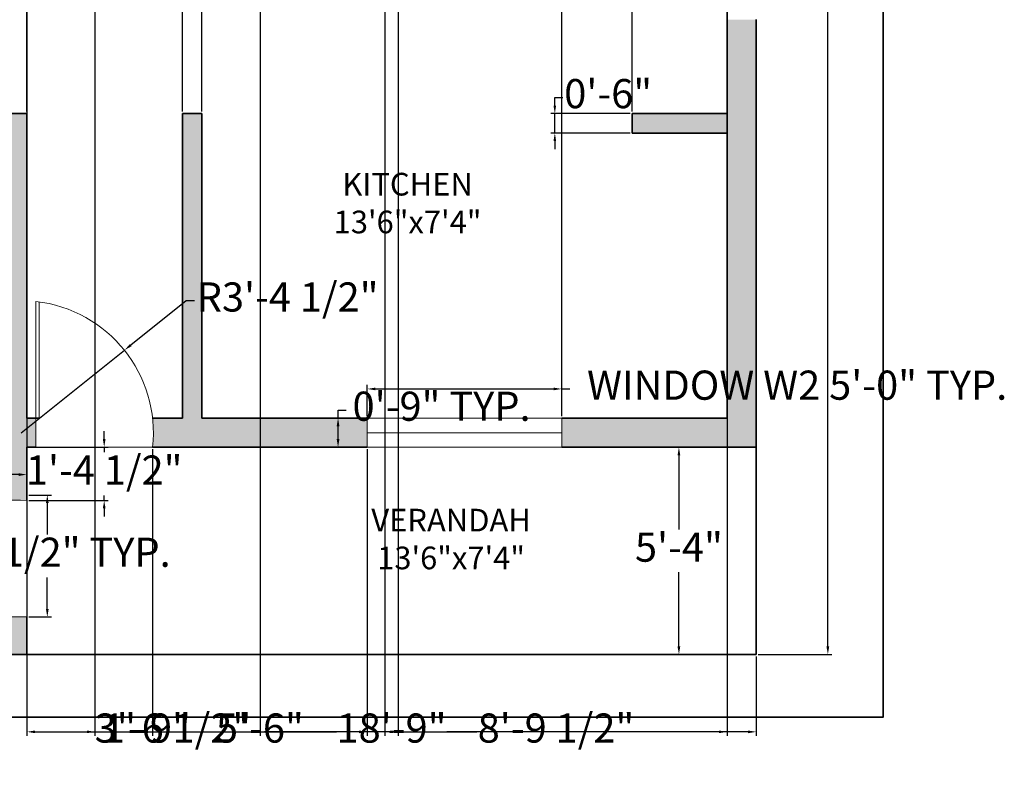
# Model space of a CAD drawing. Units: inches. Extents: x 2151 to 2709, y 3533 to 4046.
# Tile 3 of 4: x 2406 to 2709, y 3533 to 3766. Entities that reach past the tile are written whole.
import ezdxf

# ---------------------------------------------------------------- set-up
doc = ezdxf.new("R2010")
doc.units = ezdxf.units.IN
for name, color, linetype, lineweight in [('A-ANNO-DIMS', 2, 'Continuous', 18), ('A-ANNO-TTLB', 7, 'Continuous', 35), ('A-AREA-IDEN', 7, 'Continuous', 25), ('A-DOOR', 3, 'Continuous', 18), ('A-GLAZ', 4, 'Continuous', 18), ('A-WALL', 7, 'Continuous', 35)]:
    doc.layers.add(name, color=color, linetype=linetype, lineweight=lineweight)
doc.layers.add('A-WALL-PATT', color=18, linetype='Continuous', lineweight=13, true_color=0x000000)
doc.styles.get("Standard").update_dxf_attribs({"font": 'arial.ttf'})
doc.dimstyles.new('ISO-25', dxfattribs={"dimtxt": 9, "dimasz": 2.5, "dimexe": 1.25, "dimexo": 0.625, "dimgap": 2, "dimtad": 0, "dimtih": 1, "dimtoh": 1, "dimdec": 1, "dimlunit": 4, "dimtxsty": 'Standard', "dimcen": 2.5, "dimadec": 0, "dimazin": 0, "dimtfac": 0.5, "dimtdec": 1, "dimtmove": 0, "dimatfit": 3, "dimfxl": 1, "dimarcsym": 0})

# ---------------------------------------------------------------- blocks, each defined once
blk = doc.blocks.new('*D7')
at = {"layer": 'A-ANNO-DIMS', "color": 0, "lineweight": -2, "transparency": 16777216}
for p, q in [((2633.46, 4002.17), (2656.18, 4002.17)), ((2654.93, 3999.67), (2654.93, 3792.76)), ((2654.93, 3572.67), (2654.93, 3779.57)), ((2633.46, 3570.17), (2656.18, 3570.17))]:
    blk.add_line(p, q, dxfattribs=at)
at = {"layer": 'A-ANNO-DIMS', "color": 0, "transparency": 16777216}
for points in [[(2654.51, 3999.67), (2655.35, 3999.67), (2654.93, 4002.17)], [(2654.51, 3572.67), (2655.35, 3572.67), (2654.93, 3570.17)]]:
    blk.add_solid(points, dxfattribs=at)
at = {"layer": 'Defpoints', "color": 0, "transparency": 16777216}
for p in [(2632.83, 4002.17), (2632.83, 3570.17), (2654.93, 3570.17)]:
    blk.add_point(p, dxfattribs=at)
at = {"layer": 'A-ANNO-DIMS', "color": 0, "transparency": 16777216, "insert": (2654.93, 3786.17), "char_height": 9, "attachment_point": 5}
blk.add_mtext("36'", dxfattribs=at)
blk = doc.blocks.new('WIN-60IN')
for p, q in [((0, 9), (0, 0)), ((0, 9), (60, 9)), ((60, 9), (60, 0)), ((0, 4.5), (60, 4.5)), ((0, 0), (60, 0))]:
    blk.add_line(p, q)
blk = doc.blocks.new('DOOR-SWING-36IN')
for p, q in [((0, 6), (0, 42)), ((1, 6), (1, 41.91)), ((0, 6), (0, 0)), ((0, 0), (36, 0))]:
    blk.add_line(p, q)
blk.add_arc((-3, 3), 39.12, 355.6013, 85.6013)
blk = doc.blocks.new('*D15')
at = {"layer": 'A-ANNO-DIMS', "color": 0, "lineweight": -2, "transparency": 16777216}
for p, q in [((2512.83, 3643.79), (2512.83, 3653.42)), ((2515.33, 3652.17), (2570.33, 3652.17)), ((2572.83, 3643.79), (2572.83, 3653.42)), ((2572.83, 3652.17), (2575.33, 3652.17))]:
    blk.add_line(p, q, dxfattribs=at)
at = {"layer": 'A-ANNO-DIMS', "color": 0, "transparency": 16777216}
for points in [[(2515.33, 3652.58), (2515.33, 3651.75), (2512.83, 3652.17)], [(2570.33, 3652.58), (2570.33, 3651.75), (2572.83, 3652.17)]]:
    blk.add_solid(points, dxfattribs=at)
at = {"layer": 'Defpoints', "color": 0, "transparency": 16777216}
for p in [(2572.83, 3652.17), (2512.83, 3643.17), (2572.83, 3643.17)]:
    blk.add_point(p, dxfattribs=at)
at = {"layer": 'A-ANNO-DIMS', "color": 0, "transparency": 16777216, "insert": (2645.45, 3652.17), "char_height": 9, "attachment_point": 5}
blk.add_mtext('WINDOW W2 5\'-0" TYP.', dxfattribs=at)
blk = doc.blocks.new('*D16')
at = {"layer": 'A-ANNO-DIMS', "color": 0, "lineweight": -2, "transparency": 16777216}
for p, q in [((2503.83, 3643.17), (2503.83, 3645.67)), ((2503.83, 3645.67), (2506.33, 3645.67)), ((2512.21, 3643.17), (2502.58, 3643.17)), ((2503.83, 3636.67), (2503.83, 3640.67)), ((2512.21, 3634.17), (2502.58, 3634.17))]:
    blk.add_line(p, q, dxfattribs=at)
at = {"layer": 'A-ANNO-DIMS', "color": 0, "transparency": 16777216}
for points in [[(2503.41, 3640.67), (2504.25, 3640.67), (2503.83, 3643.17)], [(2503.41, 3636.67), (2504.25, 3636.67), (2503.83, 3634.17)]]:
    blk.add_solid(points, dxfattribs=at)
at = {"layer": 'Defpoints', "color": 0, "transparency": 16777216}
for p in [(2503.83, 3643.17), (2512.83, 3643.17), (2512.83, 3634.17)]:
    blk.add_point(p, dxfattribs=at)
at = {"layer": 'A-ANNO-DIMS', "color": 0, "transparency": 16777216, "insert": (2535.76, 3645.67), "char_height": 9, "attachment_point": 5}
blk.add_mtext('0\'-9" TYP.', dxfattribs=at)
blk = doc.blocks.new('*D17')
at = {"layer": 'A-ANNO-DIMS', "color": 0, "lineweight": -2, "transparency": 16777216}
for p, q in [((2365.83, 3620.05), (2365.83, 3626.98)), ((2407.83, 3620.05), (2407.83, 3626.98)), ((2365.83, 3625.73), (2363.33, 3625.73)), ((2405.33, 3625.73), (2368.33, 3625.73))]:
    blk.add_line(p, q, dxfattribs=at)
at = {"layer": 'A-ANNO-DIMS', "color": 0, "transparency": 16777216}
for points in [[(2368.33, 3626.14), (2368.33, 3625.31), (2365.83, 3625.73)], [(2405.33, 3626.14), (2405.33, 3625.31), (2407.83, 3625.73)]]:
    blk.add_solid(points, dxfattribs=at)
at = {"layer": 'Defpoints', "color": 0, "transparency": 16777216}
for p in [(2365.83, 3625.73), (2365.83, 3619.43), (2407.83, 3619.43)]:
    blk.add_point(p, dxfattribs=at)
at = {"layer": 'A-ANNO-DIMS', "color": 0, "transparency": 16777216, "insert": (2303.74, 3625.73), "char_height": 9, "attachment_point": 5}
blk.add_mtext('DOOR D1 3\'-6" TYP.', dxfattribs=at)
blk = doc.blocks.new('*D18')
at = {"layer": 'A-ANNO-DIMS', "color": 0, "lineweight": -2, "transparency": 16777216}
for p, q in [((2408.46, 3619.43), (2415.38, 3619.43)), ((2414.13, 3616.93), (2414.13, 3607.26)), ((2414.13, 3584.27), (2414.13, 3593.94)), ((2408.46, 3581.77), (2415.38, 3581.77))]:
    blk.add_line(p, q, dxfattribs=at)
at = {"layer": 'A-ANNO-DIMS', "color": 0, "transparency": 16777216}
for points in [[(2413.71, 3616.93), (2414.55, 3616.93), (2414.13, 3619.43)], [(2413.71, 3584.27), (2414.55, 3584.27), (2414.13, 3581.77)]]:
    blk.add_solid(points, dxfattribs=at)
at = {"layer": 'Defpoints', "color": 0, "transparency": 16777216}
for p in [(2407.83, 3619.43), (2414.13, 3619.43), (2407.83, 3581.77)]:
    blk.add_point(p, dxfattribs=at)
at = {"layer": 'A-ANNO-DIMS', "color": 0, "transparency": 16777216, "insert": (2414.13, 3600.6), "char_height": 9, "attachment_point": 5}
blk.add_mtext('3\'-1 1/2" TYP.', dxfattribs=at)
blk = doc.blocks.new('*D25')
at = {"layer": 'A-ANNO-DIMS', "color": 0, "lineweight": -2, "transparency": 16777216}
for p, q in [((2407.83, 3737.79), (2407.83, 4027.27)), ((2410.33, 4026.02), (2417.69, 4026.02)), ((2453.33, 4026.02), (2445.97, 4026.02)), ((2455.83, 3737.79), (2455.83, 4027.27))]:
    blk.add_line(p, q, dxfattribs=at)
at = {"layer": 'A-ANNO-DIMS', "color": 0, "transparency": 16777216}
for points in [[(2410.33, 4026.43), (2410.33, 4025.6), (2407.83, 4026.02)], [(2453.33, 4026.43), (2453.33, 4025.6), (2455.83, 4026.02)]]:
    blk.add_solid(points, dxfattribs=at)
at = {"layer": 'Defpoints', "color": 0, "transparency": 16777216}
for p in [(2455.83, 4026.02), (2407.83, 3737.17), (2455.83, 3737.17)]:
    blk.add_point(p, dxfattribs=at)
at = {"layer": 'A-ANNO-DIMS', "color": 0, "transparency": 16777216, "insert": (2431.83, 4026.02), "char_height": 9, "attachment_point": 5}
blk.add_mtext('4\'-0"', dxfattribs=at)
blk = doc.blocks.new('*D26')
at = {"layer": 'A-ANNO-DIMS', "color": 0, "lineweight": -2, "transparency": 16777216}
for p, q in [((2570.7, 3739.67), (2570.7, 3742.17)), ((2570.7, 3742.17), (2573.2, 3742.17)), ((2593.92, 3737.17), (2569.45, 3737.17)), ((2570.7, 3731.17), (2570.7, 3737.17)), ((2593.92, 3731.17), (2569.45, 3731.17)), ((2570.7, 3728.67), (2570.7, 3726.17))]:
    blk.add_line(p, q, dxfattribs=at)
at = {"layer": 'A-ANNO-DIMS', "color": 0, "transparency": 16777216}
for points in [[(2570.28, 3739.67), (2571.11, 3739.67), (2570.7, 3737.17)], [(2570.28, 3728.67), (2571.11, 3728.67), (2570.7, 3731.17)]]:
    blk.add_solid(points, dxfattribs=at)
at = {"layer": 'Defpoints', "color": 0, "transparency": 16777216}
for p in [(2570.7, 3737.17), (2594.55, 3737.17), (2594.55, 3731.17)]:
    blk.add_point(p, dxfattribs=at)
at = {"layer": 'A-ANNO-DIMS', "color": 0, "transparency": 16777216, "insert": (2587.16, 3742.17), "char_height": 9, "attachment_point": 5}
blk.add_mtext('0\'-6"', dxfattribs=at)
blk = doc.blocks.new('*D27')
at = {"layer": 'A-ANNO-DIMS', "color": 0, "lineweight": -2, "transparency": 16777216}
for p, q in [((2632.21, 3634.17), (2607.73, 3634.17)), ((2608.98, 3631.67), (2608.98, 3608.74)), ((2608.98, 3572.67), (2608.98, 3595.59)), ((2632.21, 3570.17), (2607.73, 3570.17))]:
    blk.add_line(p, q, dxfattribs=at)
at = {"layer": 'A-ANNO-DIMS', "color": 0, "transparency": 16777216}
for points in [[(2608.56, 3631.67), (2609.4, 3631.67), (2608.98, 3634.17)], [(2608.56, 3572.67), (2609.4, 3572.67), (2608.98, 3570.17)]]:
    blk.add_solid(points, dxfattribs=at)
at = {"layer": 'Defpoints', "color": 0, "transparency": 16777216}
for p in [(2608.98, 3634.17), (2632.83, 3634.17), (2632.83, 3570.17)]:
    blk.add_point(p, dxfattribs=at)
at = {"layer": 'A-ANNO-DIMS', "color": 0, "transparency": 16777216, "insert": (2608.98, 3602.17), "char_height": 9, "attachment_point": 5}
blk.add_mtext('5\'-4"', dxfattribs=at)
blk = doc.blocks.new('*D28')
at = {"layer": 'A-ANNO-DIMS', "color": 0, "lineweight": -2, "transparency": 16777216}
for p, q in [((2407.83, 3569.54), (2407.83, 3545.07)), ((2632.83, 3569.54), (2632.83, 3545.07)), ((2410.33, 3546.32), (2503.3, 3546.32)), ((2630.33, 3546.32), (2537.37, 3546.32))]:
    blk.add_line(p, q, dxfattribs=at)
at = {"layer": 'A-ANNO-DIMS', "color": 0, "transparency": 16777216}
for points in [[(2410.33, 3546.73), (2410.33, 3545.9), (2407.83, 3546.32)], [(2630.33, 3546.73), (2630.33, 3545.9), (2632.83, 3546.32)]]:
    blk.add_solid(points, dxfattribs=at)
at = {"layer": 'Defpoints', "color": 0, "transparency": 16777216}
for p in [(2407.83, 3570.17), (2632.83, 3570.17), (2632.83, 3546.32)]:
    blk.add_point(p, dxfattribs=at)
at = {"layer": 'A-ANNO-DIMS', "color": 0, "transparency": 16777216, "insert": (2520.33, 3546.32), "char_height": 9, "attachment_point": 5}
blk.add_mtext('18\'-9"', dxfattribs=at)
blk = doc.blocks.new('*D34')
at = {"layer": 'A-ANNO-DIMS', "color": 0, "lineweight": -2, "transparency": 16777216}
for p, q in [((2572.83, 3643.79), (2572.83, 4027.27)), ((2575.33, 4026.02), (2584.19, 4026.02)), ((2621.33, 4026.02), (2612.47, 4026.02)), ((2623.83, 3643.79), (2623.83, 4027.27))]:
    blk.add_line(p, q, dxfattribs=at)
at = {"layer": 'A-ANNO-DIMS', "color": 0, "transparency": 16777216}
for points in [[(2575.33, 4026.43), (2575.33, 4025.6), (2572.83, 4026.02)], [(2621.33, 4026.43), (2621.33, 4025.6), (2623.83, 4026.02)]]:
    blk.add_solid(points, dxfattribs=at)
at = {"layer": 'Defpoints', "color": 0, "transparency": 16777216}
for p in [(2623.83, 4026.02), (2572.83, 3643.17), (2623.83, 3643.17)]:
    blk.add_point(p, dxfattribs=at)
at = {"layer": 'A-ANNO-DIMS', "color": 0, "transparency": 16777216, "insert": (2598.33, 4026.02), "char_height": 9, "attachment_point": 5}
blk.add_mtext('4\'-3"', dxfattribs=at)
blk = doc.blocks.new('*D39')
at = {"layer": 'A-ANNO-DIMS', "color": 0, "lineweight": -2, "transparency": 16777216}
for p, q in [((2407.83, 3992.54), (2407.83, 3545.07)), ((2428.83, 3992.54), (2428.83, 3545.07)), ((2410.33, 3546.32), (2426.33, 3546.32)), ((2428.83, 3546.32), (2431.33, 3546.32))]:
    blk.add_line(p, q, dxfattribs=at)
at = {"layer": 'A-ANNO-DIMS', "color": 0, "transparency": 16777216}
for points in [[(2410.33, 3546.73), (2410.33, 3545.9), (2407.83, 3546.32)], [(2426.33, 3546.73), (2426.33, 3545.9), (2428.83, 3546.32)]]:
    blk.add_solid(points, dxfattribs=at)
at = {"layer": 'Defpoints', "color": 0, "transparency": 16777216}
for p in [(2407.83, 3993.17), (2428.83, 3993.17), (2428.83, 3546.32)]:
    blk.add_point(p, dxfattribs=at)
at = {"layer": 'A-ANNO-DIMS', "color": 0, "transparency": 16777216, "insert": (2444.87, 3546.32), "char_height": 9, "attachment_point": 5}
blk.add_mtext('1\'-9"', dxfattribs=at)
blk = doc.blocks.new('*D42')
at = {"layer": 'A-ANNO-DIMS', "color": 0, "lineweight": -2, "transparency": 16777216}
for p, q in [((2479.83, 3992.54), (2479.83, 3545.07)), ((2522.34, 3992.54), (2522.34, 3545.07)), ((2479.83, 3546.32), (2477.33, 3546.32)), ((2519.84, 3546.32), (2482.33, 3546.32))]:
    blk.add_line(p, q, dxfattribs=at)
at = {"layer": 'A-ANNO-DIMS', "color": 0, "transparency": 16777216}
for points in [[(2482.33, 3546.73), (2482.33, 3545.9), (2479.83, 3546.32)], [(2519.84, 3546.73), (2519.84, 3545.9), (2522.34, 3546.32)]]:
    blk.add_solid(points, dxfattribs=at)
at = {"layer": 'Defpoints', "color": 0, "transparency": 16777216}
for p in [(2479.83, 3993.17), (2522.34, 3993.17), (2479.83, 3546.32)]:
    blk.add_point(p, dxfattribs=at)
at = {"layer": 'A-ANNO-DIMS', "color": 0, "transparency": 16777216, "insert": (2452.89, 3546.32), "char_height": 9, "attachment_point": 5}
blk.add_mtext('3\'-6 1/2"', dxfattribs=at)
blk = doc.blocks.new('*D43')
at = {"layer": 'A-ANNO-DIMS', "color": 0, "lineweight": -2, "transparency": 16777216}
for p, q in [((2461.83, 3737.79), (2461.83, 4027.27)), ((2464.33, 4026.02), (2500.67, 4026.02)), ((2592.05, 4026.02), (2555.71, 4026.02)), ((2594.55, 3737.79), (2594.55, 4027.27))]:
    blk.add_line(p, q, dxfattribs=at)
at = {"layer": 'A-ANNO-DIMS', "color": 0, "transparency": 16777216}
for points in [[(2464.33, 4026.43), (2464.33, 4025.6), (2461.83, 4026.02)], [(2592.05, 4026.43), (2592.05, 4025.6), (2594.55, 4026.02)]]:
    blk.add_solid(points, dxfattribs=at)
at = {"layer": 'Defpoints', "color": 0, "transparency": 16777216}
for p in [(2594.55, 4026.02), (2461.83, 3737.17), (2594.55, 3737.17)]:
    blk.add_point(p, dxfattribs=at)
at = {"layer": 'A-ANNO-DIMS', "color": 0, "transparency": 16777216, "insert": (2528.19, 4026.02), "char_height": 9, "attachment_point": 5}
blk.add_mtext('11\'-0 1/2"', dxfattribs=at)
blk = doc.blocks.new('*D47')
at = {"layer": 'A-ANNO-DIMS', "color": 0, "lineweight": -2, "transparency": 16777216}
for p, q in [((2518.29, 3866.54), (2518.29, 3545.07)), ((2623.83, 3866.54), (2623.83, 3545.07)), ((2520.79, 3546.32), (2546.61, 3546.32)), ((2621.33, 3546.32), (2595.52, 3546.32))]:
    blk.add_line(p, q, dxfattribs=at)
at = {"layer": 'A-ANNO-DIMS', "color": 0, "transparency": 16777216}
for points in [[(2520.79, 3546.73), (2520.79, 3545.9), (2518.29, 3546.32)], [(2621.33, 3546.73), (2621.33, 3545.9), (2623.83, 3546.32)]]:
    blk.add_solid(points, dxfattribs=at)
at = {"layer": 'Defpoints', "color": 0, "transparency": 16777216}
for p in [(2518.29, 3867.17), (2623.83, 3867.17), (2623.83, 3546.32)]:
    blk.add_point(p, dxfattribs=at)
at = {"layer": 'A-ANNO-DIMS', "color": 0, "transparency": 16777216, "insert": (2571.06, 3546.32), "char_height": 9, "attachment_point": 5}
blk.add_mtext('8\'-9 1/2"', dxfattribs=at)
blk = doc.blocks.new('*D50')
at = {"layer": 'A-ANNO-DIMS', "color": 0, "lineweight": -2, "transparency": 16777216}
for p, q in [((2431.68, 3636.67), (2431.68, 3639.17)), ((2408.46, 3634.17), (2432.93, 3634.17)), ((2431.68, 3634.17), (2431.68, 3632.62)), ((2408.46, 3617.77), (2432.93, 3617.77)), ((2431.68, 3617.77), (2431.68, 3619.31)), ((2431.68, 3615.27), (2431.68, 3612.77))]:
    blk.add_line(p, q, dxfattribs=at)
at = {"layer": 'A-ANNO-DIMS', "color": 0, "transparency": 16777216}
for points in [[(2431.26, 3636.67), (2432.1, 3636.67), (2431.68, 3634.17)], [(2431.26, 3615.27), (2432.1, 3615.27), (2431.68, 3617.77)]]:
    blk.add_solid(points, dxfattribs=at)
at = {"layer": 'Defpoints', "color": 0, "transparency": 16777216}
for p in [(2407.83, 3634.17), (2407.83, 3617.77), (2431.68, 3617.77)]:
    blk.add_point(p, dxfattribs=at)
at = {"layer": 'A-ANNO-DIMS', "color": 0, "transparency": 16777216, "insert": (2431.68, 3625.97), "char_height": 9, "attachment_point": 5}
blk.add_mtext('1\'-4 1/2"', dxfattribs=at)
blk = doc.blocks.new('*D51')
at = {"layer": 'A-ANNO-DIMS', "color": 0, "lineweight": -2, "transparency": 16777216}
for p, q in [((2446.59, 3633.54), (2446.59, 3545.07)), ((2512.83, 3633.54), (2512.83, 3545.07)), ((2449.09, 3546.32), (2465.75, 3546.32)), ((2510.33, 3546.32), (2493.67, 3546.32))]:
    blk.add_line(p, q, dxfattribs=at)
at = {"layer": 'A-ANNO-DIMS', "color": 0, "transparency": 16777216}
for points in [[(2449.09, 3546.73), (2449.09, 3545.9), (2446.59, 3546.32)], [(2510.33, 3546.73), (2510.33, 3545.9), (2512.83, 3546.32)]]:
    blk.add_solid(points, dxfattribs=at)
at = {"layer": 'Defpoints', "color": 0, "transparency": 16777216}
for p in [(2446.59, 3634.17), (2512.83, 3634.17), (2512.83, 3546.32)]:
    blk.add_point(p, dxfattribs=at)
at = {"layer": 'A-ANNO-DIMS', "color": 0, "transparency": 16777216, "insert": (2479.71, 3546.32), "char_height": 9, "attachment_point": 5}
blk.add_mtext('5\'-6"', dxfattribs=at)
blk = doc.blocks.new('*D55')
at = {"layer": 'A-ANNO-DIMS', "color": 0, "lineweight": -2, "transparency": 16777216}
for p, q in [((2457, 3679.39), (2439.86, 3665.68)), ((2459.5, 3679.39), (2457, 3679.39)), ((2406.09, 3638.67), (2437.91, 3664.12))]:
    blk.add_line(p, q, dxfattribs=at)
at = {"layer": 'A-ANNO-DIMS', "color": 0, "transparency": 16777216}
blk.add_solid([(2439.6, 3666.01), (2440.12, 3665.36), (2437.91, 3664.12)], dxfattribs=at)
at = {"layer": 'Defpoints', "color": 0, "transparency": 16777216}
for p in [(2437.91, 3664.12), (2406.09, 3638.67)]:
    blk.add_point(p, dxfattribs=at)
at = {"layer": 'A-ANNO-DIMS', "color": 0, "transparency": 16777216, "insert": (2488.26, 3679.39), "char_height": 9, "attachment_point": 5}
blk.add_mtext('R3\'-4 1/2"', dxfattribs=at)

msp = doc.modelspace()

# ---------------------------------------------------------------- hatches: boundary and pattern name
at = {"layer": 'A-WALL-PATT'}
h = msp.add_hatch(color=256, dxfattribs=at)
h.dxf.hatch_style = 1
h.paths.add_polyline_path([(2461.83, 3731.17), (2461.83, 3737.17), (2455.83, 3737.17), (2455.83, 3731.17), (2455.83, 3643.17), (2446.59, 3643.17, -0.055385), (2446.59, 3634.16), (2512.83, 3634.16), (2512.83, 3643.17), (2461.83, 3643.17)])
h.paths.add_polyline_path([(2632.83, 3766.17), (2623.83, 3766.17), (2623.83, 3737.17), (2594.55, 3737.17), (2594.55, 3731.17), (2623.83, 3731.17), (2623.83, 3643.17), (2572.83, 3643.17), (2572.83, 3634.16), (2623.83, 3634.16), (2632.83, 3634.16)])
h = msp.add_hatch(color=256, dxfattribs=at)
h.dxf.hatch_style = 1
h.paths.add_polyline_path([(2407.83, 3731.17), (2407.83, 3737.17), (2400.21, 3737.17), (2400.21, 3731.17), (2401.83, 3731.17), (2401.83, 3617.77, -0.038405), (2407.83, 3617.77), (2407.83, 3634.16), (2410.59, 3634.16), (2410.59, 3643.17), (2407.83, 3643.17)])
h.paths.add_polyline_path([(2407.83, 3579.17), (2407.83, 3581.77), (2401.83, 3581.77), (2401.83, 3579.17), (2359.83, 3579.17), (2359.83, 3570.17), (2407.83, 3570.17)])

# ---------------------------------------------------------------- linework, layer by layer
at = {"layer": 'A-ANNO-TTLB'}
msp.add_lwpolyline([(2228.43, 4045.57), (2671.96, 4045.57), (2671.96, 3550.81), (2228.43, 3550.81)], close=True, dxfattribs=at)
at = {"layer": 'A-DOOR'}
for p, q in [((2410.59, 3643.17), (2410.59, 3679.17)), ((2411.59, 3643.17), (2411.59, 3679.04)), ((2410.59, 3643.17), (2410.59, 3634.16)), ((2446.59, 3634.16), (2410.59, 3634.16))]:
    msp.add_line(p, q, dxfattribs=at)
msp.add_arc((2406.09, 3638.67), 40.75, 353.6598, 83.6598, dxfattribs=at)
at = {"layer": 'A-WALL'}
for p, q in [((2623.83, 3766.17), (2623.83, 3737.17)), ((2632.83, 3766.17), (2632.83, 3570.17)), ((2400.21, 3737.17), (2407.83, 3737.17)), ((2400.21, 3737.17), (2407.83, 3737.17)), ((2407.83, 3731.17), (2407.83, 3737.17)), ((2455.83, 3737.17), (2461.83, 3737.17)), ((2455.83, 3731.17), (2455.83, 3737.17)), ((2461.83, 3731.17), (2461.83, 3737.17)), ((2594.55, 3737.17), (2594.55, 3731.17)), ((2594.55, 3737.17), (2623.83, 3737.17)), ((2594.55, 3737.17), (2594.55, 3731.17)), ((2407.83, 3643.17), (2407.83, 3731.17)), ((2455.83, 3731.17), (2455.83, 3643.17)), ((2461.83, 3731.17), (2461.83, 3643.17)), ((2594.55, 3731.17), (2623.83, 3731.17)), ((2623.83, 3731.17), (2623.83, 3643.17)), ((2407.83, 3643.17), (2411.59, 3643.17)), ((2446.59, 3643.17), (2455.83, 3643.17)), ((2461.83, 3643.17), (2512.83, 3643.17)), ((2572.83, 3643.17), (2623.83, 3643.17)), ((2407.83, 3634.16), (2410.59, 3634.16)), ((2407.83, 3617.77), (2407.83, 3634.16)), ((2446.59, 3634.16), (2512.83, 3634.16)), ((2572.83, 3634.16), (2623.83, 3634.16)), ((2623.83, 3634.16), (2632.83, 3634.16)), ((2407.83, 3579.17), (2407.83, 3581.77)), ((2407.83, 3579.17), (2407.83, 3570.17)), ((2632.83, 3570.17), (2359.83, 3570.17))]:
    msp.add_line(p, q, dxfattribs=at)

# ---------------------------------------------------------------- block references
at = {"layer": 'A-DOOR', "rotation": 89.99999999999812}
msp.add_blockref('DOOR-SWING-36IN', (2407.83, 3581.77), dxfattribs=at)
at = {"layer": 'A-GLAZ'}
msp.add_blockref('WIN-60IN', (2512.83, 3634.16), dxfattribs=at)

# ---------------------------------------------------------------- texts
at = {"layer": 'A-AREA-IDEN', "char_height": 7, "attachment_point": 1}
for s, width, insert in [('\\pxqc;{\\fArial|b1|i0|c0|p34;KITCHEN\\P13\'6"x7\'4"}', 69.8141, (2490.36, 3718.88)), ('\\pxqc;{\\fArial|b1|i0|c0|p34;VERANDAH\\P13\'6"x7\'4"}', 82.6217, (2497.38, 3615.17))]:
    msp.add_mtext_dynamic_manual_height_columns(s, width=width, gutter_width=12.5, heights=[0], dxfattribs=dict(at, insert=insert))

# ---------------------------------------------------------------- dimensions: what is measured, and where the dimension line sits
at = {"layer": 'A-ANNO-DIMS'}
for base, p1, p2, picture, middle in [((2594.55, 4026.02), (2461.83, 3737.17), (2594.55, 3737.17), '*D43', (2528.19, 4026.02)), ((2455.83, 4026.02), (2407.83, 3737.17), (2455.83, 3737.17), '*D25', (2431.83, 4026.02)), ((2623.83, 4026.02), (2572.83, 3643.17), (2623.83, 3643.17), '*D34', (2598.33, 4026.02)), ((2428.83, 3546.32), (2407.83, 3993.17), (2428.83, 3993.17), '*D39', (2444.87, 3546.32)), ((2479.83, 3546.32), (2522.34, 3993.17), (2479.83, 3993.17), '*D42', (2452.89, 3546.32)), ((2623.83, 3546.32), (2518.29, 3867.17), (2623.83, 3867.17), '*D47', (2571.06, 3546.32)), ((2512.83, 3546.32), (2446.59, 3634.16), (2512.83, 3634.16), '*D51', (2479.71, 3546.32)), ((2632.83, 3546.32), (2407.83, 3570.17), (2632.83, 3570.17), '*D28', (2520.33, 3546.32))]:
    dim = msp.add_linear_dim(base=base, p1=p1, p2=p2, dimstyle='ISO-25', override={"dimdec": 1, "dimlfac": 1, "dimrnd": 0, "dimzin": 1, "dimdsep": 46, "dimlunit": 4, "dimfrac": 2}, dxfattribs=at)
    dim.commit()
    dim.dimension.update_dxf_attribs({"geometry": picture, "text_midpoint": middle})
for base, p1, p2, angle, override, picture, middle in [((2654.93, 3570.17), (2632.83, 4002.17), (2632.83, 3570.17), 90, {"dimclrd": 0, "dimclre": 0, "dimclrt": 0}, '*D7', (2654.93, 3786.17)), ((2570.7, 3737.17), (2594.55, 3731.17), (2594.55, 3737.17), 90, {"dimdec": 1, "dimlfac": 1, "dimrnd": 0, "dimzin": 1, "dimdsep": 46, "dimlunit": 4, "dimfrac": 2}, '*D26', (2587.16, 3742.17)), ((2431.68, 3617.77), (2407.83, 3634.16), (2407.83, 3617.77), 270, {"dimdec": 1, "dimlfac": 1, "dimrnd": 0, "dimzin": 1, "dimdsep": 46, "dimlunit": 4, "dimfrac": 2}, '*D50', (2431.68, 3625.97)), ((2608.98, 3634.16), (2632.83, 3570.17), (2632.83, 3634.16), 90, {"dimdec": 1, "dimlfac": 1, "dimrnd": 0, "dimzin": 1, "dimdsep": 46, "dimlunit": 4, "dimfrac": 2}, '*D27', (2608.98, 3602.17))]:
    dim = msp.add_linear_dim(base=base, p1=p1, p2=p2, angle=angle, dimstyle='ISO-25', override=override, dxfattribs=at)
    dim.commit()
    dim.dimension.update_dxf_attribs({"geometry": picture, "text_midpoint": middle})
dim = msp.add_radius_dim(center=(2406.09, 3638.67), mpoint=(2437.91, 3664.12), dimstyle='ISO-25', override={"dimdec": 1, "dimlfac": 1, "dimrnd": 0, "dimzin": 1, "dimdsep": 46, "dimlunit": 4, "dimfrac": 2}, dxfattribs=at)
dim.commit()
dim.dimension.update_dxf_attribs({"geometry": '*D55', "text_midpoint": (2488.26, 3679.39), "dimtype": 164})
dim = msp.add_linear_dim(base=(2572.83, 3652.17), p1=(2512.83, 3643.17), p2=(2572.83, 3643.17), text='WINDOW W2 <> TYP.', dimstyle='ISO-25', override={"dimdec": 1, "dimlfac": 1, "dimrnd": 0, "dimzin": 1, "dimdsep": 46, "dimlunit": 4, "dimfrac": 2}, dxfattribs=at)
dim.commit()
dim.dimension.update_dxf_attribs({"geometry": '*D15', "text_midpoint": (2645.45, 3652.17)})
for base, p1, p2, angle, text, picture, middle in [((2503.83, 3643.17), (2512.83, 3634.16), (2512.83, 3643.17), 90, '<> TYP.', '*D16', (2535.76, 3645.67)), ((2365.83, 3625.73), (2407.83, 3619.43), (2365.83, 3619.43), 180, 'DOOR D1 <> TYP.', '*D17', (2303.74, 3625.73)), ((2414.13, 3619.43), (2407.83, 3581.77), (2407.83, 3619.43), 90, '<> TYP.', '*D18', (2414.13, 3600.6))]:
    dim = msp.add_linear_dim(base=base, p1=p1, p2=p2, angle=angle, text=text, dimstyle='ISO-25', override={"dimdec": 1, "dimlfac": 1, "dimrnd": 0, "dimzin": 1, "dimdsep": 46, "dimlunit": 4, "dimfrac": 2}, dxfattribs=at)
    dim.commit()
    dim.dimension.update_dxf_attribs({"geometry": picture, "text_midpoint": middle})

doc.saveas('drawing.dxf')
